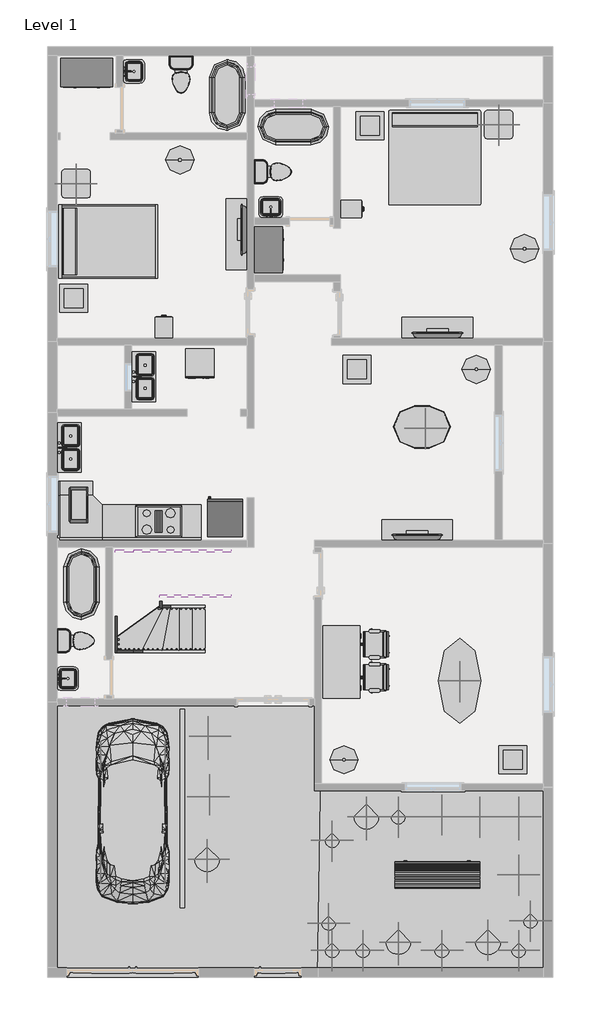
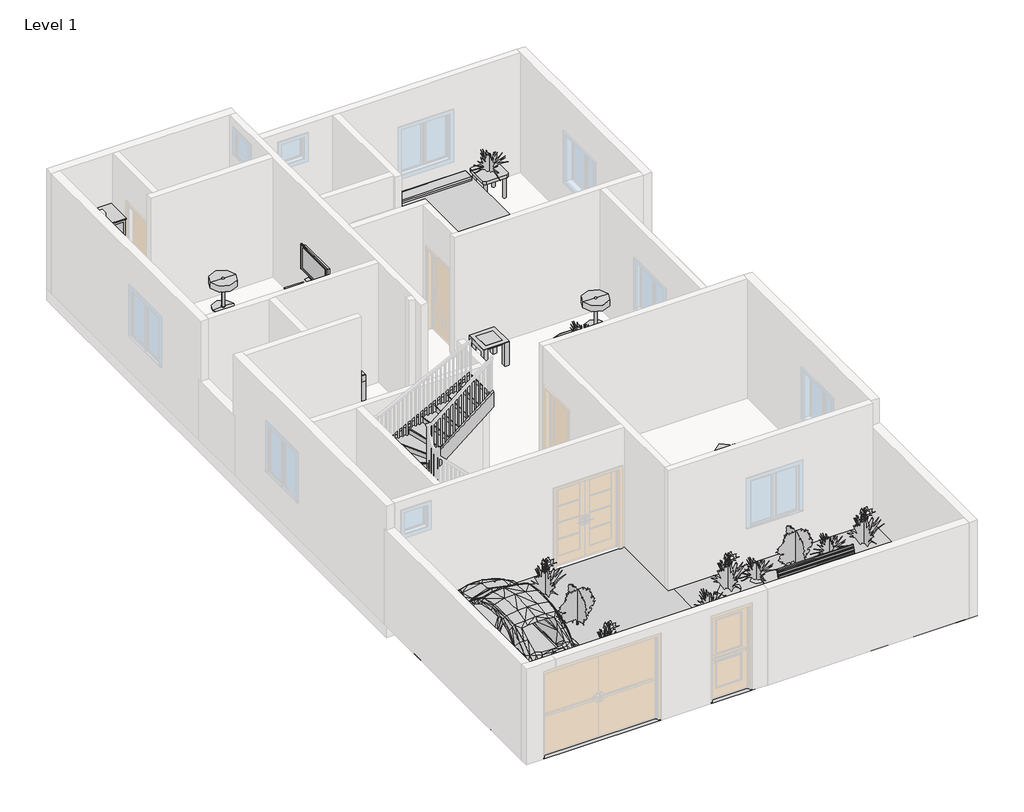
# One storey, part 3 of 3: 28 furniture elements, 23 geographic elements, 15 flow terminals, 8 members, 8 proxies, 1 stair flight.
"""IFC4 building model written with IfcOpenShell, lengths in millimetres."""

from ifc_helpers import new_model, si_unit, frame, origin, place, context, project, spatial, polyline, outline, extrude, triangles, transform, mapped, element, save
from components import proxy_bb1e6e30, proxy_45b28599, proxy_8a8d5ab2, parking_space_9_x_18_90_deg_fdd9e8f5, rpc_beetle_rpc_beetle_3ce7ba48, proxy_a13a33b2, flow_terminal_accce45a, flow_terminal_a53be723, flow_terminal_62a433f7, toilet_domestic_3d_toilet_domestic_3d_f7549cf7, toilet_domestic_3d_toilet_domestic_3d_183bbd19, flow_terminal_b374fae2, furniture_35c09872, furniture_1fc5af50, furniture_bb55ed6b, chair_task_arms_chair_task_arms_fa5a08ef, furniture_072f6425, furniture_61dbd871, furniture_f13f95b7, furniture_7a3aaa4f, furniture_b5c51a22, furniture_be1c6672, furniture_962d0db1, furniture_31d08a24, furniture_d94a64e0, furniture_3250926c, furniture_8edce76a, geographic_element_235d1464, rpc_plant_tropical_55f6ff97, rpc_plant_tropical_agave_1_5_93a2a214, rpc_plant_tropical_jungle_flame_3_9c4808c2, stair_flight_5a50a9e8

model = new_model("IFC4")

# Units and contexts
model_context = context("Model", 3, world=origin())
ifc_project = project(units=[si_unit("LENGTHUNIT", "METRE", prefix="MILLI")], contexts=[model_context])

# Site, building, storey
site = spatial("IfcSite", under=ifc_project)
building = spatial("IfcBuilding", under=site)
storey = spatial("IfcBuildingStorey", under=building, Name="Level 1", Elevation=0.0)

# Proxies
placement = place(None, origin())
element("IfcBuildingElementProxy", 1, Name="Building Element Proxy", at=placement, inside=storey, context=model_context, shape_type="Tessellation", body=[
    triangles([(-11802.0982178, -24.7005658, 0.0), (-5909.2974426, -20.372437, 0.0), (-11802.0982178, -5866.7006241, 0.0), (-6010.8976364, -5866.7006241, 0.0)], [[1, 3, 4], [4, 2, 1]], closed=False),
])
element("IfcBuildingElementProxy", 2, Name="Building Element Proxy", at=placement, inside=storey, context=model_context, shape_type="Tessellation", body=[
    triangles([(-6061.6974426, -1853.5005272, 0.0), (-6091.6241043, -5866.7006241, 0.0), (-930.8976849, -1853.5005272, 0.0), (-930.8976849, -5866.7006241, 0.0)], [[1, 2, 4], [4, 3, 1]], closed=False),
])
proxy_shape = proxy_bb1e6e30(model_context)
element("IfcBuildingElementProxy", 3, Name="Cook Top-4 Unit : 36\" x 20\"", ObjectType="Cook Top-4 Unit : 36\" x 20\"", at=placement, inside=storey, context=model_context, shape_type="MappedRepresentation", body=[
    mapped(proxy_shape, transform((-9414.4976606, 3937.699435, 0.0), x_axis=(1.0, 0.0, 0.0), y_axis=(0.0, 1.0, 0.0), z_axis=(0.0, 0.0, 1.0))),
])
proxy_2_shape = proxy_45b28599(model_context)
element("IfcBuildingElementProxy", 4, Name="Dishwasher : 24\" x 24\" x 34\"", ObjectType="Dishwasher : 24\" x 24\" x 34\"", at=placement, inside=storey, context=model_context, shape_type="MappedRepresentation", body=[
    mapped(proxy_2_shape, transform((-8907.8151291, 7074.8498702, 0.0), x_axis=(1.0, 0.0, 0.0), y_axis=(0.0, 1.0, 0.0), z_axis=(0.0, 0.0, 1.0))),
])
proxy_3_shape = proxy_8a8d5ab2(model_context)
element("IfcBuildingElementProxy", 5, Name="Microwave : 30\" x 16\" x 18\"", ObjectType="Microwave : 30\" x 16\" x 18\"", at=placement, inside=storey, context=model_context, shape_type="MappedRepresentation", body=[
    mapped(proxy_3_shape, transform((-11494.7781665, 3793.0065577, 0.0), x_axis=(0.0, 1.0, 0.0), y_axis=(-1.0, 0.0, 0.0), z_axis=(0.0, 0.0, 1.0))),
])
parking_space_9_x_18_90_deg_shape = parking_space_9_x_18_90_deg_fdd9e8f5(model_context)
element("IfcBuildingElementProxy", 6, Name="Parking Space : 9' x 18' - 90 deg", ObjectType="Parking Space : 9' x 18' - 90 deg", at=placement, inside=storey, context=model_context, shape_type="MappedRepresentation", body=[
    mapped(parking_space_9_x_18_90_deg_shape, transform((-8906.4976606, -4368.100565, 0.0), x_axis=(-1.0, 0.0, 0.0), y_axis=(0.0, -1.0, 0.0), z_axis=(0.0, 0.0, 1.0))),
])
rpc_beetle_rpc_beetle_shape = rpc_beetle_rpc_beetle_3ce7ba48(model_context)
element("IfcBuildingElementProxy", 7, Name="RPC Beetle : RPC Beetle", ObjectType="RPC Beetle : RPC Beetle", at=placement, inside=storey, context=model_context, shape_type="MappedRepresentation", body=[
    mapped(rpc_beetle_rpc_beetle_shape, transform((-9973.2976606, -3529.900565, 0.0), x_axis=(1.0, 0.0, 0.0), y_axis=(0.0, 1.0, 0.0), z_axis=(0.0, 0.0, 1.0))),
])
proxy_4_shape = proxy_a13a33b2(model_context)
element("IfcBuildingElementProxy", 8, Name="Refrigerator : 30\" x 32\" RH", ObjectType="Refrigerator : 30\" x 32\" RH", at=placement, inside=storey, context=model_context, shape_type="MappedRepresentation", body=[
    mapped(proxy_4_shape, transform((-7984.1601606, 4000.0004635, 0.0), x_axis=(-1.0000000000000004, 0.0, 0.0), y_axis=(0.0, -1.0000000000000004, 0.0), z_axis=(0.0, 0.0, 1.0))),
])

# Flow terminals
flow_terminal_shape = flow_terminal_accce45a(model_context)
element("IfcFlowTerminal", 9, ObjectType="Floor Drain - Round : 5\" Strainer - 2\" Drain", at=placement, inside=storey, context=model_context, shape_type="MappedRepresentation", body=[
    mapped(flow_terminal_shape, transform((-8474.6976606, 13716.699435, 0.0), x_axis=(1.0, 0.0, 0.0), y_axis=(0.0, 1.0, 0.0), z_axis=(0.0, 0.0, 1.0))),
])
element("IfcFlowTerminal", 10, ObjectType="Floor Drain - Round : 5\" Strainer - 2\" Drain", at=placement, inside=storey, context=model_context, shape_type="MappedRepresentation", body=[
    mapped(flow_terminal_shape, transform((-7077.6976606, 11887.899435, 0.0), x_axis=(1.0, 0.0, 0.0), y_axis=(0.0, 1.0, 0.0), z_axis=(0.0, 0.0, 1.0))),
])
element("IfcFlowTerminal", 11, ObjectType="Floor Drain - Round : 5\" Strainer - 2\" Drain", at=placement, inside=storey, context=model_context, shape_type="MappedRepresentation", body=[
    mapped(flow_terminal_shape, transform((-9160.4976606, 7341.299435, 0.0), x_axis=(1.0, 0.0, 0.0), y_axis=(0.0, 1.0, 0.0), z_axis=(0.0, 0.0, 1.0))),
])
element("IfcFlowTerminal", 12, ObjectType="Floor Drain - Round : 5\" Strainer - 2\" Drain", at=placement, inside=storey, context=model_context, shape_type="MappedRepresentation", body=[
    mapped(flow_terminal_shape, transform((-10709.8976606, 1753.299435, 0.0), x_axis=(1.0, 0.0, 0.0), y_axis=(0.0, 1.0, 0.0), z_axis=(0.0, 0.0, 1.0))),
])
flow_terminal_2_shape = flow_terminal_a53be723(model_context)
element("IfcFlowTerminal", 13, ObjectType="Sink Kitchen-Double : 42\" x 21\"", at=placement, inside=storey, context=model_context, shape_type="MappedRepresentation", body=[
    mapped(flow_terminal_2_shape, transform((-9742.3522595, 7033.5101944, 0.0), x_axis=(0.0, 1.0, 0.0), y_axis=(-1.0, 0.0, 0.0), z_axis=(0.0, 0.0, 1.0))),
])
element("IfcFlowTerminal", 14, ObjectType="Sink Kitchen-Double : 42\" x 21\"", at=placement, inside=storey, context=model_context, shape_type="MappedRepresentation", body=[
    mapped(flow_terminal_2_shape, transform((-11342.5522595, 5509.5101944, 0.0), x_axis=(0.0, 1.0000000000000002, 0.0), y_axis=(-1.0000000000000002, 0.0, 0.0), z_axis=(0.0, 0.0, 1.0))),
])
flow_terminal_3_shape = flow_terminal_62a433f7(model_context)
element("IfcFlowTerminal", 15, ObjectType="Sink Vanity-Square : 20\" x 18\"", at=placement, inside=storey, context=model_context, shape_type="MappedRepresentation", body=[
    mapped(flow_terminal_3_shape, transform((-9996.3522595, 13599.4101944, 0.0), x_axis=(0.0, 1.0, 0.0), y_axis=(-1.0, 0.0, 0.0), z_axis=(0.0, 0.0, 1.0))),
])
element("IfcFlowTerminal", 16, ObjectType="Sink Vanity-Square : 20\" x 18\"", at=placement, inside=storey, context=model_context, shape_type="MappedRepresentation", body=[
    mapped(flow_terminal_3_shape, transform((-6985.8084201, 10645.6448361, 0.0), x_axis=(-1.0000000000000002, 0.0, 0.0), y_axis=(0.0, -1.0000000000000002, 0.0), z_axis=(0.0, 0.0, 1.0))),
])
element("IfcFlowTerminal", 17, ObjectType="Sink Vanity-Square : 20\" x 18\"", at=placement, inside=storey, context=model_context, shape_type="MappedRepresentation", body=[
    mapped(flow_terminal_3_shape, transform((-11418.7522595, 543.8101944, 0.0), x_axis=(0.0, 1.0, 0.0), y_axis=(-1.0, 0.0, 0.0), z_axis=(0.0, 0.0, 1.0))),
])
toilet_domestic_3d_toilet_domestic_3d_shape = toilet_domestic_3d_toilet_domestic_3d_f7549cf7(model_context)
toilet_domestic_3d_toilet_domestic_3d_2_shape = toilet_domestic_3d_toilet_domestic_3d_183bbd19(model_context)
element("IfcFlowTerminal", 18, ObjectType="Toilet-Domestic-3D : Toilet-Domestic-3D", at=placement, inside=storey, context=model_context, shape_type="MappedRepresentation", body=[
    mapped(toilet_domestic_3d_toilet_domestic_3d_shape, transform((-8931.8976606, 13450.6034076, 0.0), x_axis=(1.0, 0.0, 0.0), y_axis=(0.0, 1.0, 0.0), z_axis=(0.0, 0.0, 1.0))),
    mapped(toilet_domestic_3d_toilet_domestic_3d_2_shape, transform((-8931.8976606, 13450.6034076, 0.0), x_axis=(1.0, 0.0, 0.0), y_axis=(0.0, 1.0, 0.0), z_axis=(0.0, 0.0, 1.0))),
])
element("IfcFlowTerminal", 19, ObjectType="Toilet-Domestic-3D : Toilet-Domestic-3D", at=placement, inside=storey, context=model_context, shape_type="MappedRepresentation", body=[
    mapped(toilet_domestic_3d_toilet_domestic_3d_shape, transform((-6862.4016333, 11456.099435, 0.0), x_axis=(0.0, 1.0000000000000002, 0.0), y_axis=(-1.0000000000000002, 0.0, 0.0), z_axis=(0.0, 0.0, 1.0))),
    mapped(toilet_domestic_3d_toilet_domestic_3d_2_shape, transform((-6862.4016333, 11456.099435, 0.0), x_axis=(0.0, 1.0000000000000002, 0.0), y_axis=(-1.0000000000000002, 0.0, 0.0), z_axis=(0.0, 0.0, 1.0))),
])
element("IfcFlowTerminal", 20, ObjectType="Toilet-Domestic-3D : Toilet-Domestic-3D", at=placement, inside=storey, context=model_context, shape_type="MappedRepresentation", body=[
    mapped(toilet_domestic_3d_toilet_domestic_3d_shape, transform((-11104.2016333, 1372.299435, 0.0), x_axis=(0.0, 1.0000000000000002, 0.0), y_axis=(-1.0000000000000002, 0.0, 0.0), z_axis=(0.0, 0.0, 1.0))),
    mapped(toilet_domestic_3d_toilet_domestic_3d_2_shape, transform((-11104.2016333, 1372.299435, 0.0), x_axis=(0.0, 1.0000000000000002, 0.0), y_axis=(-1.0000000000000002, 0.0, 0.0), z_axis=(0.0, 0.0, 1.0))),
])
flow_terminal_4_shape = flow_terminal_b374fae2(model_context)
element("IfcFlowTerminal", 21, ObjectType="Tub-Free Standing-3D : 30\" x 60\"", at=placement, inside=storey, context=model_context, shape_type="MappedRepresentation", body=[
    mapped(flow_terminal_4_shape, transform((-7941.2976606, 13107.099435, 0.0), x_axis=(-1.0, 0.0, 0.0), y_axis=(0.0, -1.0, 0.0), z_axis=(0.0, 0.0, 1.0))),
])
element("IfcFlowTerminal", 22, ObjectType="Tub-Free Standing-3D : 30\" x 60\"", at=placement, inside=storey, context=model_context, shape_type="MappedRepresentation", body=[
    mapped(flow_terminal_4_shape, transform((-6518.8976606, 12421.299435, 0.0), x_axis=(0.0, -1.0000000000000004, 0.0), y_axis=(1.0000000000000004, 0.0, 0.0), z_axis=(0.0, 0.0, 1.0))),
])
element("IfcFlowTerminal", 23, ObjectType="Tub-Free Standing-3D : 30\" x 60\"", at=placement, inside=storey, context=model_context, shape_type="MappedRepresentation", body=[
    mapped(flow_terminal_4_shape, transform((-11077.0779843, 2585.7534076, 0.0), x_axis=(1.0, 0.0, 0.0), y_axis=(0.0, 1.0, 0.0), z_axis=(0.0, 0.0, 1.0))),
])

# Furniture
furniture_shape = furniture_35c09872(model_context)
element("IfcFurniture", 24, ObjectType="Bed-Shaker : Queen 62\" x 83\"", at=placement, inside=storey, context=model_context, shape_type="MappedRepresentation", body=[
    mapped(furniture_shape, transform((-11548.0976606, 9976.549435, 0.0), x_axis=(0.0, 1.0000000000000002, 0.0), y_axis=(-1.0000000000000002, 0.0, 0.0), z_axis=(0.0, 0.0, 1.0))),
])
furniture_2_shape = furniture_1fc5af50(model_context)
element("IfcFurniture", 25, ObjectType="Bed-Standard : King 78\" x 80\"", at=placement, inside=storey, context=model_context, shape_type="MappedRepresentation", body=[
    mapped(furniture_2_shape, transform((-3742.3861852, 11806.494517, 0.0), x_axis=(1.0, 0.0, 0.0), y_axis=(0.0, 1.0, 0.0), z_axis=(0.0, 0.0, 1.0))),
])
furniture_3_shape = furniture_bb55ed6b(model_context)
element("IfcFurniture", 26, ObjectType="Cabinet-File 2 Drawer : 15\" x 18\"", at=placement, inside=storey, context=model_context, shape_type="MappedRepresentation", body=[
    mapped(furniture_3_shape, transform((-9428.0941077, 7961.1651349, 0.0), x_axis=(-0.9999999999999998, 0.0, 0.0), y_axis=(0.0, -0.9999999999999998, 0.0), z_axis=(0.0, 0.0, 1.0))),
])
element("IfcFurniture", 27, ObjectType="Cabinet-File 2 Drawer : 15\" x 18\"", at=placement, inside=storey, context=model_context, shape_type="MappedRepresentation", body=[
    mapped(furniture_3_shape, transform((-5416.4319608, 10783.895882, 0.0), x_axis=(0.0, 1.0, 0.0), y_axis=(-1.0, 0.0, 0.0), z_axis=(0.0, 0.0, 1.0))),
])
chair_task_arms_chair_task_arms_shape = chair_task_arms_chair_task_arms_fa5a08ef(model_context)
element("IfcFurniture", 28, ObjectType="Chair-Task Arms : Chair-Task Arms", at=placement, inside=storey, context=model_context, shape_type="MappedRepresentation", body=[
    mapped(chair_task_arms_chair_task_arms_shape, transform((-4721.951759, 1155.1086153, 0.0), x_axis=(0.0, 1.0000000000000009, 0.0), y_axis=(-1.0000000000000009, 0.0, 0.0), z_axis=(0.0, 0.0, 1.0))),
])
element("IfcFurniture", 29, ObjectType="Chair-Task Arms : Chair-Task Arms", at=placement, inside=storey, context=model_context, shape_type="MappedRepresentation", body=[
    mapped(chair_task_arms_chair_task_arms_shape, transform((-4721.951759, 443.9086153, 0.0), x_axis=(0.0, 1.0000000000000002, 0.0), y_axis=(-1.0000000000000002, 0.0, 0.0), z_axis=(0.0, 0.0, 1.0))),
])
furniture_4_shape = furniture_072f6425(model_context)
element("IfcFurniture", 30, ObjectType="Desk : 60\" x 30\" Student", at=placement, inside=storey, context=model_context, shape_type="MappedRepresentation", body=[
    mapped(furniture_4_shape, transform((-5858.4976606, 1677.099435, 0.0), x_axis=(0.0, -1.0000000000000004, 0.0), y_axis=(1.0000000000000004, 0.0, 0.0), z_axis=(0.0, 0.0, 1.0))),
])
furniture_5_shape = furniture_61dbd871(model_context)
element("IfcFurniture", 31, ObjectType="Dresser : 48\" x 72\" x 24\"", at=placement, inside=storey, context=model_context, shape_type="MappedRepresentation", body=[
    mapped(furniture_5_shape, transform((-10694.7044008, 13952.8623891, 0.0), x_axis=(1.0, 0.0, 0.0), y_axis=(0.0, 1.0, 0.0), z_axis=(0.0, 0.0, 1.0))),
])
furniture_6_shape = furniture_f13f95b7(model_context)
element("IfcFurniture", 32, ObjectType="Dresser : 48\" x 72\" x 24\" 2", at=placement, inside=storey, context=model_context, shape_type="MappedRepresentation", body=[
    mapped(furniture_6_shape, transform((-7415.4606147, 10048.8926948, 0.0), x_axis=(0.0, 1.0000000000000002, 0.0), y_axis=(-1.0000000000000002, 0.0, 0.0), z_axis=(0.0, 0.0, 1.0))),
])
furniture_7_shape = furniture_7a3aaa4f(model_context)
element("IfcFurniture", 33, ObjectType="TV - Flat Screen : 42\"", at=placement, inside=storey, context=model_context, shape_type="MappedRepresentation", body=[
    mapped(furniture_7_shape, transform((-7568.0362843, 10207.5549208, 1041.4), x_axis=(0.0, -1.0000000000000002, 0.0), y_axis=(1.0000000000000002, 0.0, 0.0), z_axis=(0.0, 0.0, 1.0))),
])
element("IfcFurniture", 34, ObjectType="TV - Flat Screen : 42\"", at=placement, inside=storey, context=model_context, shape_type="MappedRepresentation", body=[
    mapped(furniture_7_shape, transform((-3417.6921748, 7933.2380586, 1041.4), x_axis=(-0.9999999999999998, 0.0, 0.0), y_axis=(0.0, -0.9999999999999998, 0.0), z_axis=(0.0, 0.0, 1.0))),
])
element("IfcFurniture", 35, ObjectType="TV - Flat Screen : 42\"", at=placement, inside=storey, context=model_context, shape_type="MappedRepresentation", body=[
    mapped(furniture_7_shape, transform((-3855.8421748, 3589.8380586, 1041.4), x_axis=(-1.0000000000000004, 0.0, 0.0), y_axis=(0.0, -1.0000000000000004, 0.0), z_axis=(0.0, 0.0, 1.0))),
])
furniture_8_shape = furniture_b5c51a22(model_context)
element("IfcFurniture", 36, ObjectType="Table-Coffee : 24\" x 24\" x 24\"", at=placement, inside=storey, context=model_context, shape_type="MappedRepresentation", body=[
    mapped(furniture_8_shape, transform((-11261.5634273, 8643.0883572, 0.0), x_axis=(1.0, 0.0, 0.0), y_axis=(0.0, 1.0, 0.0), z_axis=(0.0, 0.0, 1.0))),
])
element("IfcFurniture", 37, ObjectType="Table-Coffee : 24\" x 24\" x 24\"", at=placement, inside=storey, context=model_context, shape_type="MappedRepresentation", body=[
    mapped(furniture_8_shape, transform((-4886.1634273, 12351.4883572, 0.0), x_axis=(1.0, 0.0, 0.0), y_axis=(0.0, 1.0, 0.0), z_axis=(0.0, 0.0, 1.0))),
])
element("IfcFurniture", 38, ObjectType="Table-Coffee : 24\" x 24\" x 24\"", at=placement, inside=storey, context=model_context, shape_type="MappedRepresentation", body=[
    mapped(furniture_8_shape, transform((-5165.5634273, 7112.7383572, 0.0), x_axis=(1.0, 0.0, 0.0), y_axis=(0.0, 1.0, 0.0), z_axis=(0.0, 0.0, 1.0))),
])
element("IfcFurniture", 39, ObjectType="Table-Coffee : 24\" x 24\" x 24\"", at=placement, inside=storey, context=model_context, shape_type="MappedRepresentation", body=[
    mapped(furniture_8_shape, transform((-1812.7634273, -1281.9616428, 0.0), x_axis=(1.0, 0.0, 0.0), y_axis=(0.0, 1.0, 0.0), z_axis=(0.0, 0.0, 1.0))),
])
furniture_9_shape = furniture_be1c6672(model_context)
element("IfcFurniture", 40, ObjectType="Table-Dining Oval : 36\" x 48\"", at=placement, inside=storey, context=model_context, shape_type="MappedRepresentation", body=[
    mapped(furniture_9_shape, transform((-4152.1173328, 5611.6010743, 0.0), x_axis=(-1.0000000000000002, 0.0, 0.0), y_axis=(0.0, -1.0000000000000002, 0.0), z_axis=(0.0, 0.0, 1.0))),
])
furniture_10_shape = furniture_962d0db1(model_context)
element("IfcFurniture", 41, ObjectType="Table-Ellipse : 72\" x 36\"", at=placement, inside=storey, context=model_context, shape_type="MappedRepresentation", body=[
    mapped(furniture_10_shape, transform((-2937.4976606, 508.699435, 0.0), x_axis=(0.0, 1.0000000000000002, 0.0), y_axis=(-1.0000000000000002, 0.0, 0.0), z_axis=(0.0, 0.0, 1.0))),
])
furniture_11_shape = furniture_31d08a24(model_context)
element("IfcFurniture", 42, ObjectType="Table-End : 24\" x 24\"", at=placement, inside=storey, context=model_context, shape_type="MappedRepresentation", body=[
    mapped(furniture_11_shape, transform((-11501.0312909, 11049.699435, 0.0), x_axis=(1.0, 0.0, 0.0), y_axis=(0.0, 1.0, 0.0), z_axis=(0.0, 0.0, 1.0))),
])
element("IfcFurniture", 43, ObjectType="Table-End : 24\" x 24\"", at=placement, inside=storey, context=model_context, shape_type="MappedRepresentation", body=[
    mapped(furniture_11_shape, transform((-2407.8312909, 12319.699435, 0.0), x_axis=(1.0, 0.0, 0.0), y_axis=(0.0, 1.0, 0.0), z_axis=(0.0, 0.0, 1.0))),
])
furniture_12_shape = furniture_d94a64e0(model_context)
element("IfcFurniture", 44, ObjectType="Table-Rectangular : 72\" x 30\"", at=placement, inside=storey, context=model_context, shape_type="MappedRepresentation", body=[
    mapped(furniture_12_shape, transform((-7738.0976606, 10109.899435, 0.0), x_axis=(0.0, 1.0000000000000002, 0.0), y_axis=(-1.0000000000000002, 0.0, 0.0), z_axis=(0.0, 0.0, 1.0))),
])
element("IfcFurniture", 45, ObjectType="Table-Rectangular : 72\" x 30\"", at=placement, inside=storey, context=model_context, shape_type="MappedRepresentation", body=[
    mapped(furniture_12_shape, transform((-3413.7476606, 8103.299435, 0.0), x_axis=(1.0, 0.0, 0.0), y_axis=(0.0, 1.0, 0.0), z_axis=(0.0, 0.0, 1.0))),
])
element("IfcFurniture", 46, ObjectType="Table-Rectangular : 72\" x 30\"", at=placement, inside=storey, context=model_context, shape_type="MappedRepresentation", body=[
    mapped(furniture_12_shape, transform((-3851.8976606, 3741.299435, 0.0), x_axis=(1.0, 0.0, 0.0), y_axis=(0.0, 1.0, 0.0), z_axis=(0.0, 0.0, 1.0))),
])
furniture_13_shape = furniture_3250926c(model_context)
element("IfcFurniture", 47, ObjectType="Table-Round : 36\" Diameter", at=placement, inside=storey, context=model_context, shape_type="MappedRepresentation", body=[
    mapped(furniture_13_shape, transform((-8957.2976606, 11710.099435, 0.0), x_axis=(1.0, 0.0, 0.0), y_axis=(0.0, 1.0, 0.0), z_axis=(0.0, 0.0, 1.0))),
])
element("IfcFurniture", 48, ObjectType="Table-Round : 36\" Diameter", at=placement, inside=storey, context=model_context, shape_type="MappedRepresentation", body=[
    mapped(furniture_13_shape, transform((-1540.4976606, 9805.099435, 0.0), x_axis=(1.0, 0.0, 0.0), y_axis=(0.0, 1.0, 0.0), z_axis=(0.0, 0.0, 1.0))),
])
element("IfcFurniture", 49, ObjectType="Table-Round : 36\" Diameter", at=placement, inside=storey, context=model_context, shape_type="MappedRepresentation", body=[
    mapped(furniture_13_shape, transform((-2581.8976606, 7207.949435, 0.0), x_axis=(1.0, 0.0, 0.0), y_axis=(0.0, 1.0, 0.0), z_axis=(0.0, 0.0, 1.0))),
])
element("IfcFurniture", 50, ObjectType="Table-Round : 36\" Diameter", at=placement, inside=storey, context=model_context, shape_type="MappedRepresentation", body=[
    mapped(furniture_13_shape, transform((-5426.6976606, -1186.750565, 0.0), x_axis=(1.0, 0.0, 0.0), y_axis=(0.0, 1.0, 0.0), z_axis=(0.0, 0.0, 1.0))),
])
furniture_14_shape = furniture_8edce76a(model_context)
element("IfcFurniture", 51, ObjectType="Work Station Cubicle : 96\" x 96\"", at=placement, inside=storey, context=model_context, shape_type="MappedRepresentation", body=[
    mapped(furniture_14_shape, transform((-12093.9206683, 3663.0311872, 0.0), x_axis=(0.0, 1.0000000000000009, 0.0), y_axis=(-1.0000000000000009, 0.0, 0.0), z_axis=(0.0, 0.0, 1.0))),
])

# Geographic elements
geographic_element_shape = geographic_element_235d1464(model_context)
element("IfcGeographicElement", 52, ObjectType="Park Bench : 72\"", at=placement, inside=storey, context=model_context, shape_type="MappedRepresentation", body=[
    mapped(geographic_element_shape, transform((-3420.0976606, -3631.500565, 0.0), x_axis=(1.0, 0.0, 0.0), y_axis=(0.0, 1.0, 0.0), z_axis=(0.0, 0.0, 1.0))),
])
rpc_plant_tropical_shape = rpc_plant_tropical_55f6ff97(model_context)
element("IfcGeographicElement", 53, ObjectType="RPC Plant - Tropical", at=placement, inside=storey, context=model_context, shape_type="MappedRepresentation", body=[
    mapped(rpc_plant_tropical_shape, transform((-8347.6976606, -685.100565, 0.0), x_axis=(1.0, 0.0, 0.0), y_axis=(0.0, 1.0, 0.0), z_axis=(0.0, 0.0, 1.0))),
])
element("IfcGeographicElement", 54, ObjectType="RPC Plant - Tropical", at=placement, inside=storey, context=model_context, shape_type="MappedRepresentation", body=[
    mapped(rpc_plant_tropical_shape, transform((-8373.0976606, -3326.700565, 0.0), x_axis=(1.0, 0.0, 0.0), y_axis=(0.0, 1.0, 0.0), z_axis=(0.0, 0.0, 1.0))),
])
element("IfcGeographicElement", 55, ObjectType="RPC Plant - Tropical", at=placement, inside=storey, context=model_context, shape_type="MappedRepresentation", body=[
    mapped(rpc_plant_tropical_shape, transform((-1667.4976606, -2412.300565, 0.0), x_axis=(1.0, 0.0, 0.0), y_axis=(0.0, 1.0, 0.0), z_axis=(0.0, 0.0, 1.0))),
])
element("IfcGeographicElement", 56, ObjectType="RPC Plant - Tropical", at=placement, inside=storey, context=model_context, shape_type="MappedRepresentation", body=[
    mapped(rpc_plant_tropical_shape, transform((-4944.0976606, -2412.300565, 0.0), x_axis=(1.0, 0.0, 0.0), y_axis=(0.0, 1.0, 0.0), z_axis=(0.0, 0.0, 1.0))),
])
element("IfcGeographicElement", 57, ObjectType="RPC Plant - Tropical", at=placement, inside=storey, context=model_context, shape_type="MappedRepresentation", body=[
    mapped(rpc_plant_tropical_shape, transform((-4258.2976606, -5104.700565, 0.0), x_axis=(1.0, 0.0, 0.0), y_axis=(0.0, 1.0, 0.0), z_axis=(0.0, 0.0, 1.0))),
])
rpc_plant_tropical_agave_1_5_shape = rpc_plant_tropical_agave_1_5_93a2a214(model_context)
element("IfcGeographicElement", 58, ObjectType="RPC Plant - Tropical : Agave - 1.5'", at=placement, inside=storey, context=model_context, shape_type="MappedRepresentation", body=[
    mapped(rpc_plant_tropical_agave_1_5_shape, transform((-11192.4976606, 11202.099435, 609.6), x_axis=(1.0, 0.0, 0.0), y_axis=(0.0, 1.0, 0.0), z_axis=(0.0, 0.0, 1.0))),
])
element("IfcGeographicElement", 59, ObjectType="RPC Plant - Tropical : Agave - 1.5'", at=placement, inside=storey, context=model_context, shape_type="MappedRepresentation", body=[
    mapped(rpc_plant_tropical_agave_1_5_shape, transform((-2099.2976606, 12472.099435, 609.6), x_axis=(1.0, 0.0, 0.0), y_axis=(0.0, 1.0, 0.0), z_axis=(0.0, 0.0, 1.0))),
])
element("IfcGeographicElement", 60, ObjectType="RPC Plant - Tropical : Agave - 1.5'", at=placement, inside=storey, context=model_context, shape_type="MappedRepresentation", body=[
    mapped(rpc_plant_tropical_agave_1_5_shape, transform((-3674.0976606, 5944.299435, 736.6), x_axis=(1.0, 0.0, 0.0), y_axis=(0.0, 1.0, 0.0), z_axis=(0.0, 0.0, 1.0))),
])
element("IfcGeographicElement", 61, ObjectType="RPC Plant - Tropical : Agave - 1.5'", at=placement, inside=storey, context=model_context, shape_type="MappedRepresentation", body=[
    mapped(rpc_plant_tropical_agave_1_5_shape, transform((-2937.4976606, 508.699435, 660.4), x_axis=(1.0, 0.0, 0.0), y_axis=(0.0, 1.0, 0.0), z_axis=(0.0, 0.0, 1.0))),
])
element("IfcGeographicElement", 62, ObjectType="RPC Plant - Tropical : Agave - 1.5'", at=placement, inside=storey, context=model_context, shape_type="MappedRepresentation", body=[
    mapped(rpc_plant_tropical_agave_1_5_shape, transform((-5680.6976606, -5282.500565, 0.0), x_axis=(1.0, 0.0, 0.0), y_axis=(0.0, 1.0, 0.0), z_axis=(0.0, 0.0, 1.0))),
])
element("IfcGeographicElement", 63, ObjectType="RPC Plant - Tropical : Agave - 1.5'", at=placement, inside=storey, context=model_context, shape_type="MappedRepresentation", body=[
    mapped(rpc_plant_tropical_agave_1_5_shape, transform((-5020.2976606, -5282.500565, 0.0), x_axis=(1.0, 0.0, 0.0), y_axis=(0.0, 1.0, 0.0), z_axis=(0.0, 0.0, 1.0))),
])
element("IfcGeographicElement", 64, ObjectType="RPC Plant - Tropical : Agave - 1.5'", at=placement, inside=storey, context=model_context, shape_type="MappedRepresentation", body=[
    mapped(rpc_plant_tropical_agave_1_5_shape, transform((-3318.4976606, -5282.500565, 0.0), x_axis=(1.0, 0.0, 0.0), y_axis=(0.0, 1.0, 0.0), z_axis=(0.0, 0.0, 1.0))),
])
element("IfcGeographicElement", 65, ObjectType="RPC Plant - Tropical : Agave - 1.5'", at=placement, inside=storey, context=model_context, shape_type="MappedRepresentation", body=[
    mapped(rpc_plant_tropical_agave_1_5_shape, transform((-1667.4976606, -5282.500565, 0.0), x_axis=(1.0, 0.0, 0.0), y_axis=(0.0, 1.0, 0.0), z_axis=(0.0, 0.0, 1.0))),
])
element("IfcGeographicElement", 66, ObjectType="RPC Plant - Tropical : Agave - 1.5'", at=placement, inside=storey, context=model_context, shape_type="MappedRepresentation", body=[
    mapped(rpc_plant_tropical_agave_1_5_shape, transform((-1667.4976606, -3656.900565, 0.0), x_axis=(1.0, 0.0, 0.0), y_axis=(0.0, 1.0, 0.0), z_axis=(0.0, 0.0, 1.0))),
])
element("IfcGeographicElement", 67, ObjectType="RPC Plant - Tropical : Agave - 1.5'", at=placement, inside=storey, context=model_context, shape_type="MappedRepresentation", body=[
    mapped(rpc_plant_tropical_agave_1_5_shape, transform((-1413.4976606, -4647.500565, 0.0), x_axis=(1.0, 0.0, 0.0), y_axis=(0.0, 1.0, 0.0), z_axis=(0.0, 0.0, 1.0))),
])
element("IfcGeographicElement", 68, ObjectType="RPC Plant - Tropical : Agave - 1.5'", at=placement, inside=storey, context=model_context, shape_type="MappedRepresentation", body=[
    mapped(rpc_plant_tropical_agave_1_5_shape, transform((-4258.2976606, -2412.300565, 0.0), x_axis=(1.0, 0.0, 0.0), y_axis=(0.0, 1.0, 0.0), z_axis=(0.0, 0.0, 1.0))),
])
element("IfcGeographicElement", 69, ObjectType="RPC Plant - Tropical : Agave - 1.5'", at=placement, inside=storey, context=model_context, shape_type="MappedRepresentation", body=[
    mapped(rpc_plant_tropical_agave_1_5_shape, transform((-2505.6976606, -2412.300565, 0.0), x_axis=(1.0, 0.0, 0.0), y_axis=(0.0, 1.0, 0.0), z_axis=(0.0, 0.0, 1.0))),
])
element("IfcGeographicElement", 70, ObjectType="RPC Plant - Tropical : Agave - 1.5'", at=placement, inside=storey, context=model_context, shape_type="MappedRepresentation", body=[
    mapped(rpc_plant_tropical_agave_1_5_shape, transform((-5680.6976606, -2920.300565, 0.0), x_axis=(1.0, 0.0, 0.0), y_axis=(0.0, 1.0, 0.0), z_axis=(0.0, 0.0, 1.0))),
])
element("IfcGeographicElement", 71, ObjectType="RPC Plant - Tropical : Agave - 1.5'", at=placement, inside=storey, context=model_context, shape_type="MappedRepresentation", body=[
    mapped(rpc_plant_tropical_agave_1_5_shape, transform((-5756.8976606, -4698.300565, 0.0), x_axis=(1.0, 0.0, 0.0), y_axis=(0.0, 1.0, 0.0), z_axis=(0.0, 0.0, 1.0))),
])
rpc_plant_tropical_jungle_flame_3_shape = rpc_plant_tropical_jungle_flame_3_9c4808c2(model_context)
element("IfcGeographicElement", 72, ObjectType="RPC Plant - Tropical : Jungle Flame - 3'", at=placement, inside=storey, context=model_context, shape_type="MappedRepresentation", body=[
    mapped(rpc_plant_tropical_jungle_flame_3_shape, transform((-8322.2976606, -1980.500565, 0.0), x_axis=(1.0, 0.0, 0.0), y_axis=(0.0, 1.0, 0.0), z_axis=(0.0, 0.0, 1.0))),
])
element("IfcGeographicElement", 73, ObjectType="RPC Plant - Tropical : Jungle Flame - 3'", at=placement, inside=storey, context=model_context, shape_type="MappedRepresentation", body=[
    mapped(rpc_plant_tropical_jungle_flame_3_shape, transform((-3318.4976606, -2412.300565, 0.0), x_axis=(1.0, 0.0, 0.0), y_axis=(0.0, 1.0, 0.0), z_axis=(0.0, 0.0, 1.0))),
])
element("IfcGeographicElement", 74, ObjectType="RPC Plant - Tropical : Jungle Flame - 3'", at=placement, inside=storey, context=model_context, shape_type="MappedRepresentation", body=[
    mapped(rpc_plant_tropical_jungle_flame_3_shape, transform((-2327.8976606, -5104.700565, 0.0), x_axis=(1.0, 0.0, 0.0), y_axis=(0.0, 1.0, 0.0), z_axis=(0.0, 0.0, 1.0))),
])

# Members
element("IfcMember", 75, ObjectType="Stringer - 2\" Width", at=placement, inside=storey, context=model_context, shape_type="SweptSolid", body=[
    extrude(outline(polyline([(241.2701641, -8420.1659688), (577.8751786, -8420.1659688), (1301.9005649, -9965.2595296), (965.2955504, -9965.2595296), (241.2701641, -8420.1659688)])), frame((0.0, 1118.299435, 0.0), z_axis=(0.0, 1.0, 0.0), x_axis=(0.0, 0.0, 1.0)), (0.0, 0.0, 1.0), 50.8),
])
element("IfcMember", 76, ObjectType="Stringer - 2\" Width", at=placement, inside=storey, context=model_context, shape_type="SweptSolid", body=[
    extrude(outline(polyline([(-9965.2595296, 1169.099435), (-9965.2595296, 1118.299435), (-10303.4976606, 1118.299435), (-10303.4976606, 1169.099435), (-9965.2595296, 1169.099435)])), frame((0.0, 0.0, 965.2955504), z_axis=(0.0, 0.0, 1.0), x_axis=(1.0, 0.0, 0.0)), (0.0, 0.0, 1.0), 336.6050145),
])
element("IfcMember", 77, ObjectType="Stringer - 2\" Width", at=placement, inside=storey, context=model_context, shape_type="SweptSolid", body=[
    extrude(outline(polyline([(1118.299435, 997.1005649), (1118.299435, 1285.6001408), (3251.2116775, 1969.9972697), (3277.299435, 1969.9972697), (3277.299435, 1641.7631511), (1268.2192323, 997.1005649), (1118.299435, 997.1005649)])), frame((-10354.2976606, 0.0, 0.0), z_axis=(1.0, 0.0, 0.0), x_axis=(0.0, 1.0, 0.0)), (0.0, 0.0, 1.0), 50.8),
])
element("IfcMember", 78, ObjectType="Stringer - 2\" Width", at=placement, inside=storey, context=model_context, shape_type="SweptSolid", body=[
    extrude(outline(polyline([(-10354.2976606, 3277.299435), (-10354.2976606, 3328.099435), (-9948.7831605, 3328.099435), (-9948.7831605, 3277.299435), (-10354.2976606, 3277.299435)])), frame((0.0, 0.0, 1649.8904473), z_axis=(0.0, 0.0, 1.0), x_axis=(1.0, 0.0, 0.0)), (0.0, 0.0, 1.0), 320.1068224),
])
element("IfcMember", 79, ObjectType="Stringer - 2\" Width", at=placement, inside=storey, context=model_context, shape_type="SweptSolid", body=[
    extrude(outline(polyline([(1969.9972697, -9948.7831605), (1649.8904473, -9948.7831605), (2725.6461385, -7861.3659688), (3045.7529609, -7861.3659688), (1969.9972697, -9948.7831605)])), frame((0.0, 3277.299435, 0.0), z_axis=(0.0, 1.0, 0.0), x_axis=(0.0, 0.0, 1.0)), (0.0, 0.0, 1.0), 50.8),
])
element("IfcMember", 80, ObjectType="Stringer - 2\" Width", at=placement, inside=storey, context=model_context, shape_type="SweptSolid", body=[
    extrude(outline(polyline([(61.3897561, -8420.1659688), (489.3391875, -8420.1659688), (1394.2045547, -9338.2976606), (966.2551233, -9338.2976606), (61.3897561, -8420.1659688)])), frame((0.0, 2083.499435, 0.0), z_axis=(0.0, 1.0, 0.0), x_axis=(0.0, 0.0, 1.0)), (0.0, 0.0, 1.0), 50.8),
])
element("IfcMember", 81, ObjectType="Stringer - 2\" Width", at=placement, inside=storey, context=model_context, shape_type="SweptSolid", body=[
    extrude(outline(polyline([(2083.499435, 1016.3211008), (2083.499435, 1573.2682978), (2290.1365524, 1926.1409689), (2312.099435, 1926.1409689), (2312.099435, 1360.465107), (2110.5736971, 1016.3211008), (2083.499435, 1016.3211008)])), frame((-9389.0976606, 0.0, 0.0), z_axis=(1.0, 0.0, 0.0), x_axis=(0.0, 1.0, 0.0)), (0.0, 0.0, 1.0), 50.8),
])
element("IfcMember", 82, ObjectType="Stringer - 2\" Width", at=placement, inside=storey, context=model_context, shape_type="SweptSolid", body=[
    extrude(outline(polyline([(1926.1409689, -9389.0976606), (1532.8634131, -9389.0976606), (2778.5262875, -7861.3659688), (3171.8038432, -7861.3659688), (1926.1409689, -9389.0976606)])), frame((0.0, 2312.099435, 0.0), z_axis=(0.0, 1.0, 0.0), x_axis=(0.0, 0.0, 1.0)), (0.0, 0.0, 1.0), 50.8),
])

# Stair flight
stair_flight_shape = stair_flight_5a50a9e8(model_context)
element("IfcStairFlight", 83, ObjectType="2\" Tread 1\" Nosing 1/4\" Riser", at=placement, inside=storey, context=model_context, shape_type="MappedRepresentation", body=[
    mapped(stair_flight_shape, transform((0.0, 0.0, 0.0), x_axis=(1.0, 0.0, 0.0), y_axis=(0.0, 1.0, 0.0), z_axis=(0.0, 0.0, 1.0))),
])

save(model, "model.ifc")

# Revit data of these elements
# Type "Cook Top-4 Unit : 36\" x 20\""
#   Assembly Code = "E1090400"
#   Depth = 2' - 0"
#   Width = 3' - 0"
#   Burner Material = Steel, Chrome Plated
#   Cooktop Material = Steel, Polished
#   Default Elevation = 0
# Type "Dishwasher : 24\" x 24\" x 34\""
#   Label = "DW"
#   Assembly Code = "E1090400"
#   Depth = 2' - 0"
#   Height = 2' - 10"
#   Width = 2' - 0"
#   Dishwasher Material = Steel, Paint Finish, Ivory, Glossy
#   Panel Face Material = Plastic, Opaque Black
#   Default Elevation = 0
# Type "Microwave : 30\" x 16\" x 18\""
#   Assembly Code = "E1090400"
#   Depth = 1' - 4"
#   Height = 1' - 6"
#   Width = 2' - 6"
#   Microwave Material = Laminate, Linen, Matte
#   Default Elevation = 0
# Type "Parking Space : 9' x 18' - 90 deg"
#   Angle = 90.00°
#   Parking Length = 18' - 0"
#   Parking Width = 9' - 0"
#   pl = 14' - 0"
#   pw = 7' - 0"
# Type "RPC Beetle : RPC Beetle"
#   built-in parameter 1005195 = "RPC-16-0U6E-L4EG-ENH1-J3KF-SVEL-0TX4-C0"
#   Height = 0
# Type "Refrigerator : 30\" x 32\" RH"
#   Label = "REF."
#   Assembly Code = "E1090400"
#   Depth = 2' - 7 3/4"
#   Handle = 2' - 3"
#   Height = 5' - 10"
#   Rear Clearance = 0' - 2"
#   Top Door Height = 1' - 8"
#   Width = 2' - 5 3/8"
#   Material = Carpet (1)
#   Default Elevation = 0
# Type "Floor Drain - Round : 5\" Strainer - 2\" Drain"
#   WFU = 2
#   Strainer Height = 0' - 3 1/4"
#   Strainer Radius = 0' - 2 1/2"
#   Strainer Diameter = 0' - 5"
#   Radius 6 = 0' - 0 5/8"
#   Radius 5 = 0' - 1 1/4"
#   Radius 4 = 0' - 1 7/8"
#   Radius 2 = 0' - 3.04167"
#   Radius 1 = 0' - 2.02083"
#   Radius 3 = 0' - 2 1/32"
#   Pipe Radius = 1"
#   Pipe Diameter = 2"
#   Height 2 = 0' - 0.725"
#   Height 1 = 0' - 1 13/16"
#   Body Radius = 0' - 4 1/16"
#   Body Height = 0' - 3 5/8"
#   Body Diameter = 0' - 8 1/8"
#   Drain Material = none
#   HWFU = 0
#   Default Elevation = 0
#   CWFU = 0
# Type "Sink Kitchen-Double : 42\" x 21\""
#   Assembly Code = "D2010410"
#   Counter Height = 3' - 0"
#   Depth = 1' - 9"
#   Width = 3' - 6"
#   Faucet Material = Steel, Polished
#   Sink Material = Steel, Polished
#   Default Elevation = 0
# Type "Sink Vanity-Square : 20\" x 18\""
#   Assembly Code = "D2010400"
#   Counter Height = 2' - 7"
#   Depth = 1' - 6"
#   Width = 1' - 8"
#   Basin Material = Porcelain, Linen
#   Faucet Material = Steel, Polished
#   Default Elevation = 0
# Type "Toilet-Domestic-3D : Toilet-Domestic-3D"
#   Assembly Code = "D2010110"
#   Toilet - Bowl/Basin Material = Porcelain, Linen
#   Toilet - Seat Material = Laminate, Linen, Matte
#   Default Elevation = 0
# Type "Tub-Free Standing-3D : 30\" x 60\""
#   Assembly Code = "D2010110"
#   Height = 1' - 6"
#   Length = 5' - 0"
#   Width = 2' - 6"
#   Tub Material = Porcelain, Ivory
#   Default Elevation = 0
# Type "Bed-Shaker : Queen 62\" x 83\""
#   Assembly Code = "E2020200"
#   Length = 6' - 11"
#   Width = 5' - 2"
#   Frame Material = Birch
#   Mattress Material = Plywood, Sheathing
#   Default Elevation = 0
# Type "Bed-Standard : King 78\" x 80\""
#   Assembly Code = "E2020200"
#   Length = 6' - 8"
#   Width = 6' - 6"
#   Leg Material = Steel, Chrome Plated
#   Mattress Material = Linen, White
#   Default Elevation = 0
# Type "Cabinet-File 2 Drawer : 15\" x 18\""
#   Assembly Code = "E2020200"
#   Depth = 1' - 6"
#   Height = 2' - 5"
#   Width = 1' - 3"
#   Cabinet Material = Steel, Paint Finish, Ivory, Glossy
#   Handle Material = Steel, Chrome Plated
#   Default Elevation = 0
# Type "Chair-Task Arms : Chair-Task Arms"
#   Assembly Code = "E2020200"
#   Base Material = Plastic, Opaque Black
#   Caster Material = Plastic, Opaque Black
#   Seat/Back Material = Textile - Slate Blue
#   Default Elevation = 0
# Type "Desk : 60\" x 30\" Student"
#   Assembly Code = "E2020200"
#   Depth = 2' - 6"
#   Height = 2' - 6"
#   Leg Height = 0' - 6"
#   Width = 5' - 0"
#   Body Material = Laminate, Ivory, Matte
#   Handle/Leg Material = Steel, Chrome Plated
#   Top Material = Cherry
#   Default Elevation = 0
# Type "Dresser : 48\" x 72\" x 24\""
#   Assembly Code = "E2020200"
#   Depth = 2' - 0"
#   Height = 6' - 0"
#   Width = 3' - 8"
#   Dresser Material = Wood Door Panel - Birch
#   Drawer Material = Wood Door Panel - Birch
#   Knob Material = Cherry
#   Default Elevation = 0
# Type "Dresser : 48\" x 72\" x 24\" 2"
#   Assembly Code = "E2020200"
#   Depth = 2' - 0"
#   Height = 6' - 0"
#   Width = 3' - 3"
#   Dresser Material = Wood Door Panel - Birch
#   Drawer Material = Wood Door Panel - Birch
#   Knob Material = Cherry
#   Default Elevation = 0
# Type "TV - Flat Screen : 42\""
#   SinAng = 0' - 0.0193"
#   L = 3' - 0.71517"
#   H = 1' - 8.65418"
#   Thickness = 0' - 4.33071"
#   Diagonal = 3' - 6.12598"
#   CosAng = 0' - 0.03431"
#   Stand [instance default] = yes
#   Default Elevation = 0
# Type "Table-Coffee : 24\" x 24\" x 24\""
#   Assembly Code = "E2020200"
#   Height = 2' - 0"
#   Length = 2' - 0"
#   Width = 2' - 0"
#   Top Material = none
#   Frame Material = none
#   Default Elevation = 0
# Type "Table-Dining Oval : 36\" x 48\""
#   Assembly Code = "E2020200"
#   Length = 4' - 0"
#   Width = 3' - 0"
#   Base Material = Steel, Chrome Plated
#   Top Material = Glass - Clear, Grey
#   Default Elevation = 0
#   Description = (empty or 0)
# Type "Table-Ellipse : 72\" x 36\""
#   Assembly Code = "E2020200"
#   Half Width = 1' - 6"
#   Half Length = 3' - 0"
#   Height = 2' - 2"
#   Length = 6' - 0"
#   Width = 3' - 0"
#   Base Material = Birch
#   Top Material = Sash
#   Default Elevation = 0
# Type "Table-End : 24\" x 24\""
#   Assembly Code = "E2020200"
#   Height = 2' - 0"
#   Length = 2' - 0"
#   Width = 2' - 0"
#   Base Material = Birch
#   Top Material = Laminate, Ivory, Matte
#   Default Elevation = 0
# Type "Table-Rectangular : 72\" x 30\""
#   Assembly Code = "E2020200"
#   Height = 2' - 2"
#   Length = 5' - 0"
#   Width = 1' - 6"
#   Base Material = Birch
#   Top Material = Birch
#   Default Elevation = 0
# Type "Table-Round : 36\" Diameter"
#   Assembly Code = "E2020200"
#   Base Radius = 0' - 10"
#   Height = 2' - 0"
#   Radius = 1' - 0"
#   Base Material = Steel, Chrome Plated
#   Top Material = Birch
#   Default Elevation = 0
# Type "Work Station Cubicle : 96\" x 96\""
#   Assembly Code = "E2020"
#   Desktop Height = 2' - 6"
#   Desktop1 Width = 2' - 4"
#   Desktop2 Width = 2' - 4"
#   Panel Height = 2' - 8"
#   Panel1 Length = 7' - 0"
#   Panel2 Length = 1' - 0"
#   Cube Panel Material = Textile - Light Gray
#   Work Top Material = Laminate, Ivory, Matte
#   Default Elevation = 0
# Type "Park Bench : 72\""
#   Length = 6' - 0"
#   Seat Material = Wood - Teak
#   Frame Material = Steel, Paint Finish, Dark Gray, Matte
# Type "RPC Plant - Tropical"
#   built-in parameter 1005198 = "{2, 15},{39, RPC-16-FWM5-GM7X-C67P-4000-ST1L-LVER-AU},{1, 0},{1, 0},{2, 13},{1, 8},{5, Color},{1, 0},{1, 0},{3, 0.8},{3, 0.8},{3, 0.8},{1, 8},{7, BBoxMin},{1, 0},{1, 0},{1, 0},{1, 0},{1, 0},{1, 8},{7, BBoxMax},{1, 0},{1, 0},{1, 0},{1, 0},{1, 0},{2, 11},{9, RPCTypeId},{1, 0},{1, 0},{39, RPC-16-FWM5-GM7X-C67P-4000-ST1L-LVER-AU},{1, 6},{14, RPCPlantHeight},{1, 0},{1, 0},{1, 3},{2, 11},{7, keyword},{1, 0},{1, 0},{35, :RPCs:Shrubs [General]:Geometry:RPC},{2, 11},{8, category},{1, 0},{1, 0},{16, Shrubs [General]},{2, 11},{12, LocalizedUID},{1, 0},{1, 0},{10, Crane Lily},{2, 14},{6, Height},{1, 0},{1, 0},{1, 3},{1, 2},{16, Cast Reflections},{1, 0},{1, 0},{1, 0},{1, 2},{12, Cast Shadows},{1, 0},{1, 0},{1, 1},{1, 2},{9, Lock View},{1, 0},{1, 0},{1, 0},{1, 4},{5, ViewC},{1, 0},{1, 0},{1, 0},{21, assetlibrary_base.fbx},{1, 5},"
#   built-in parameter 1005195 = "RPC-16-FWM5-GM7X-C67P-4000-ST1L-LVER-AU"
#   Assembly Code = "G2050500"
#   Height = 3' - 0"
#   Default Elevation = 0
# Type "RPC Plant - Tropical : Agave - 1.5'"
#   built-in parameter 1005198 = "{2, 15},{39, RPC-16-G1GJ-63FX-7K5P-N000-ST1L-LVER-AU},{1, 0},{1, 0},{2, 13},{1, 8},{5, Color},{1, 0},{1, 0},{3, 0.8},{3, 0.8},{3, 0.8},{1, 8},{7, BBoxMin},{1, 0},{1, 0},{1, 0},{1, 0},{1, 0},{1, 8},{7, BBoxMax},{1, 0},{1, 0},{1, 0},{1, 0},{1, 0},{2, 11},{9, RPCTypeId},{1, 0},{1, 0},{39, RPC-16-G1GJ-63FX-7K5P-N000-ST1L-LVER-AU},{1, 6},{14, RPCPlantHeight},{1, 0},{1, 0},{3, 1.5},{2, 11},{7, keyword},{1, 0},{1, 0},{35, :RPCs:Plants [General]:Geometry:RPC},{2, 11},{8, category},{1, 0},{1, 0},{16, Plants [General]},{2, 11},{12, LocalizedUID},{1, 0},{1, 0},{5, Agave},{2, 14},{6, Height},{1, 0},{1, 0},{3, 1.5},{1, 2},{16, Cast Reflections},{1, 0},{1, 0},{1, 0},{1, 2},{12, Cast Shadows},{1, 0},{1, 0},{1, 1},{1, 2},{9, Lock View},{1, 0},{1, 0},{1, 0},{1, 4},{5, ViewC},{1, 0},{1, 0},{1, 0},{21, assetlibrary_base.fbx},{1, 5},"
#   built-in parameter 1005195 = "RPC-16-G1GJ-63FX-7K5P-N000-ST1L-LVER-AU"
#   Type Comments = "Agave"
#   Assembly Code = "G2050500"
#   Height = 1' - 6"
#   Default Elevation = 0
# Type "RPC Plant - Tropical : Jungle Flame - 3'"
#   built-in parameter 1005198 = "{2, 15},{39, RPC-16-FUVJ-JWG0-MWGK-8000-ST1L-LVER-AU},{1, 0},{1, 0},{2, 13},{1, 8},{5, Color},{1, 0},{1, 0},{3, 0.8},{3, 0.8},{3, 0.8},{1, 8},{7, BBoxMin},{1, 0},{1, 0},{1, 0},{1, 0},{1, 0},{1, 8},{7, BBoxMax},{1, 0},{1, 0},{1, 0},{1, 0},{1, 0},{2, 11},{9, RPCTypeId},{1, 0},{1, 0},{39, RPC-16-FUVJ-JWG0-MWGK-8000-ST1L-LVER-AU},{1, 6},{14, RPCPlantHeight},{1, 0},{1, 0},{1, 3},{2, 11},{7, keyword},{1, 0},{1, 0},{35, :RPCs:Shrubs [General]:Geometry:RPC},{2, 11},{8, category},{1, 0},{1, 0},{16, Shrubs [General]},{2, 11},{12, LocalizedUID},{1, 0},{1, 0},{12, Jungle Flame},{2, 14},{6, Height},{1, 0},{1, 0},{1, 3},{1, 2},{16, Cast Reflections},{1, 0},{1, 0},{1, 0},{1, 2},{12, Cast Shadows},{1, 0},{1, 0},{1, 1},{1, 2},{9, Lock View},{1, 0},{1, 0},{1, 0},{1, 4},{5, ViewC},{1, 0},{1, 0},{1, 0},{21, assetlibrary_base.fbx},{1, 5},"
#   built-in parameter 1005195 = "RPC-16-FUVJ-JWG0-MWGK-8000-ST1L-LVER-AU"
#   Type Comments = "Jungle Flame"
#   Assembly Code = "G2050500"
#   Height = 3' - 0"
#   Default Elevation = 0
# Elements 1, 2 (IfcBuildingElementProxy)
#   Material = Plant
#   Phase Created = New Construction
# Element 3 (IfcBuildingElementProxy, "Cook Top-4 Unit : 36\" x 20\"")
#   Phase Created = New Construction
#   Materials on its faces: "Steel, Chrome Plated", "Steel, Polished"
# Element 4 (IfcBuildingElementProxy, "Dishwasher : 24\" x 24\" x 34\"")
#   Phase Created = New Construction
#   Materials on its faces: "Steel, Paint Finish, Ivory, Glossy", "Plastic, Opaque Black"
# Element 5 (IfcBuildingElementProxy, "Microwave : 30\" x 16\" x 18\"")
#   Phase Created = New Construction
#   Materials on its faces: "Laminate, Linen, Matte", "Glass"
# Element 6 (IfcBuildingElementProxy, "Parking Space : 9' x 18' - 90 deg")
#   Phase Created = New Construction
#   Materials on its faces: "Parking Stripe"
# Element 7 (IfcBuildingElementProxy, "RPC Beetle : RPC Beetle")
#   Phase Created = New Construction
# Element 8 (IfcBuildingElementProxy, "Refrigerator : 30\" x 32\" RH")
#   Phase Created = New Construction
#   Materials on its faces: "Carpet (1)", "Steel, Chrome Plated"
# Element 9 (IfcFlowTerminal, "Floor Drain - Round : 5\" Strainer - 2\" Drain")
#   Mark = "4"
#   Phase Created = New Construction
# Element 10 (IfcFlowTerminal, "Floor Drain - Round : 5\" Strainer - 2\" Drain")
#   Mark = "8"
#   Phase Created = New Construction
# Element 11 (IfcFlowTerminal, "Floor Drain - Round : 5\" Strainer - 2\" Drain")
#   Mark = "10"
#   Phase Created = New Construction
# Element 12 (IfcFlowTerminal, "Floor Drain - Round : 5\" Strainer - 2\" Drain")
#   Mark = "14"
#   Phase Created = New Construction
# Element 13 (IfcFlowTerminal, "Sink Kitchen-Double : 42\" x 21\"")
#   Mark = "9"
#   Phase Created = New Construction
#   Materials on its faces: "Steel, Polished"
# Element 14 (IfcFlowTerminal, "Sink Kitchen-Double : 42\" x 21\"")
#   Mark = "11"
#   Phase Created = New Construction
#   Materials on its faces: "Steel, Polished"
# Element 15 (IfcFlowTerminal, "Sink Vanity-Square : 20\" x 18\"")
#   Mark = "1"
#   Phase Created = New Construction
#   Materials on its faces: "Porcelain, Linen", "Steel, Polished"
# Element 16 (IfcFlowTerminal, "Sink Vanity-Square : 20\" x 18\"")
#   Mark = "6"
#   Phase Created = New Construction
#   Materials on its faces: "Porcelain, Linen", "Steel, Polished"
# Element 17 (IfcFlowTerminal, "Sink Vanity-Square : 20\" x 18\"")
#   Mark = "13"
#   Phase Created = New Construction
#   Materials on its faces: "Porcelain, Linen", "Steel, Polished"
# Element 18 (IfcFlowTerminal, "Toilet-Domestic-3D : Toilet-Domestic-3D")
#   Mark = "3"
#   Phase Created = New Construction
#   Materials on its faces: "Porcelain, Linen", "Laminate, Linen, Matte"
# Element 19 (IfcFlowTerminal, "Toilet-Domestic-3D : Toilet-Domestic-3D")
#   Mark = "7"
#   Phase Created = New Construction
#   Materials on its faces: "Porcelain, Linen", "Laminate, Linen, Matte"
# Element 20 (IfcFlowTerminal, "Toilet-Domestic-3D : Toilet-Domestic-3D")
#   Mark = "16"
#   Phase Created = New Construction
#   Materials on its faces: "Porcelain, Linen", "Laminate, Linen, Matte"
# Element 21 (IfcFlowTerminal, "Tub-Free Standing-3D : 30\" x 60\"")
#   Mark = "2"
#   Phase Created = New Construction
#   Materials on its faces: "Porcelain, Ivory"
# Element 22 (IfcFlowTerminal, "Tub-Free Standing-3D : 30\" x 60\"")
#   Mark = "5"
#   Phase Created = New Construction
#   Materials on its faces: "Porcelain, Ivory"
# Element 23 (IfcFlowTerminal, "Tub-Free Standing-3D : 30\" x 60\"")
#   Mark = "15"
#   Phase Created = New Construction
#   Materials on its faces: "Porcelain, Ivory"
# Element 24 (IfcFurniture, "Bed-Shaker : Queen 62\" x 83\"")
#   Phase Created = New Construction
#   Materials on its faces: "Birch", "Plywood, Sheathing"
# Element 25 (IfcFurniture, "Bed-Standard : King 78\" x 80\"")
#   Phase Created = New Construction
#   Materials on its faces: "Linen, White", "Steel, Chrome Plated"
# Elements 26, 27 (IfcFurniture, "Cabinet-File 2 Drawer : 15\" x 18\"")
#   Phase Created = New Construction
#   Materials on its faces: "Steel, Chrome Plated", "Steel, Paint Finish, Ivory, Glossy"
# Elements 28, 29 (IfcFurniture, "Chair-Task Arms : Chair-Task Arms")
#   Phase Created = New Construction
#   Materials on its faces: "Plastic, Opaque Black", "Textile - Slate Blue"
# Element 30 (IfcFurniture, "Desk : 60\" x 30\" Student")
#   Phase Created = New Construction
#   Materials on its faces: "Steel, Chrome Plated", "Laminate, Ivory, Matte", "Cherry"
# Element 31 (IfcFurniture, "Dresser : 48\" x 72\" x 24\"")
#   Phase Created = New Construction
#   Materials on its faces: "Laminate, Ivory, Matte", "Cherry", "Wood Door Panel - Birch"
# Element 32 (IfcFurniture, "Dresser : 48\" x 72\" x 24\" 2")
#   Phase Created = New Construction
#   Materials on its faces: "Laminate, Ivory, Matte", "Cherry", "Wood Door Panel - Birch"
# Elements 33, 34, 35 (IfcFurniture, "TV - Flat Screen : 42\"")
#   Stand = yes
#   Phase Created = New Construction
#   Materials on its faces: "TV - Black", "TV - Glass", "TV - Screen"
# Elements 36, 37, 38, 39 (IfcFurniture, "Table-Coffee : 24\" x 24\" x 24\"")
#   Phase Created = New Construction
#   Materials on its faces: "Glass - Clear, Grey"
# Element 40 (IfcFurniture, "Table-Dining Oval : 36\" x 48\"")
#   Phase Created = New Construction
#   Materials on its faces: "Steel, Chrome Plated", "Glass - Clear, Grey"
# Element 41 (IfcFurniture, "Table-Ellipse : 72\" x 36\"")
#   Phase Created = New Construction
#   Materials on its faces: "Birch", "Sash"
# Elements 42, 43 (IfcFurniture, "Table-End : 24\" x 24\"")
#   Phase Created = New Construction
#   Materials on its faces: "Laminate, Ivory, Matte", "Birch"
# Elements 44, 45, 46 (IfcFurniture, "Table-Rectangular : 72\" x 30\"")
#   Phase Created = New Construction
#   Materials on its faces: "Birch"
# Elements 47, 48, 49, 50 (IfcFurniture, "Table-Round : 36\" Diameter")
#   Phase Created = New Construction
#   Materials on its faces: "Steel, Chrome Plated", "Birch"
# Element 51 (IfcFurniture, "Work Station Cubicle : 96\" x 96\"")
#   Phase Created = New Construction
#   Materials on its faces: "Textile - Light Gray", "Laminate, Ivory, Matte"
# Element 52 (IfcGeographicElement, "Park Bench : 72\"")
#   Phase Created = New Construction
#   Materials on its faces: "Wood - Teak", "Steel, Paint Finish, Dark Gray, Matte"
# Elements 53, 54, 55, 56, 57 (IfcGeographicElement, "RPC Plant - Tropical")
#   Phase Created = New Construction
# Elements 58, 59, 60, 61, 62, 63, 64, 65, 66, 67, 68, 69, 70, 71 (IfcGeographicElement, "RPC Plant - Tropical : Agave - 1.5'")
#   Phase Created = New Construction
# Elements 72, 73, 74 (IfcGeographicElement, "RPC Plant - Tropical : Jungle Flame - 3'")
#   Phase Created = New Construction
# Elements 75, 76, 77, 78, 79, 80, 81, 82 (IfcMember, "Stringer - 2\" Width")
#   Phase Created = New Construction
# Element 83 (IfcStairFlight, "2\" Tread 1\" Nosing 1/4\" Riser")
#   Phase Created = New Construction
# Materials
#   "Steel, Chrome Plated": class "Metal", colour RGB 17 17 17, transparency 0, Description = "Chromiuim plated steel", Cost = 0
#   "Steel, Polished": class "Metal", colour RGB 57 57 57, transparency 0, Description = "Polished steel", Cost = 0
#   "Steel, Paint Finish, Ivory, Glossy": class "Metal", colour RGB 247 247 239, transparency 0, Description = "Steel, paint finish, ivory, glossy", Cost = 0
#   "Plastic, Opaque Black": class "Plastic", colour RGB 0 0 0, transparency 0.7, Description = "Plastic, generic, opaque black", Cost = 0
#   "Laminate, Linen, Matte": class "Plastic", colour RGB 249 239 230, transparency 0, Description = "Plastic Laminate - Linen, Matte", Cost = 0
#   "Carpet (1)": class "Carpet", colour RGB 124 80 67, transparency 0, Description = "Interior finish"
#   "Porcelain, Linen": class "Ceramic", colour RGB 249 239 230, transparency 0, Description = "Porcelain, linen", Cost = 0
#   "Porcelain, Ivory": class "Ceramic", colour RGB 247 247 239, transparency 0, Description = "Porcelain, ivory", Cost = 0
#   "Birch": class "Wood", colour RGB 210 159 95, transparency 0, Description = "Betula Alleghaniensis", Cost = 0
#   "Plywood, Sheathing": class "Wood", colour RGB 212 179 113, transparency 0, Description = "Plywood, sheathing grade", Cost = 0
#   "Linen, White": class "Textile", colour RGB 247 247 239, transparency 0, Description = "Linen, white", Cost = 0
#   "Textile - Slate Blue": class "Fabric", colour RGB 98 102 118, transparency 0
#   "Laminate, Ivory, Matte": class "Plastic", colour RGB 247 247 239, transparency 0, Description = "Plastic Laminate - Ivory, Matte", Cost = 0
#   "Cherry": class "Wood", colour RGB 226 177 128, transparency 0, Description = "Prunus Serotina", Cost = 0
#   "Wood Door Panel - Birch": class "Wood", colour RGB 166 116 52, transparency 0
#   "Glass - Clear, Grey": class "Glass", colour RGB 252 255 255, transparency 0.64
#   "Sash": class "Wood", colour RGB 224 178 126, transparency 0
#   "Textile - Light Gray": class "Fabric", colour RGB 204 204 204, transparency 0
#   "Wood - Teak": class "Wood", colour RGB 145 112 90, transparency 0
#   "Steel, Paint Finish, Dark Gray, Matte": class "Metal", colour RGB 0 0 0, transparency 0, Description = "Steel, paint finish, dark gray, matte", Cost = 0
#   "Plant": class "Generic", colour RGB 0 0 0, transparency 0, Description = "physical material", Cost = 0
#   "Glass": class "Glass", colour RGB 0 128 192, transparency 0.75, Description = "Soda Lime Glass", Cost = 0
#   "Parking Stripe": class "Paint", colour RGB 250 250 91, transparency 0
#   "TV - Black": colour RGB 49 49 49, transparency 0
#   "TV - Glass": colour RGB 157 157 157, transparency 0.9
#   "TV - Screen": colour RGB 0 0 0, transparency 0
